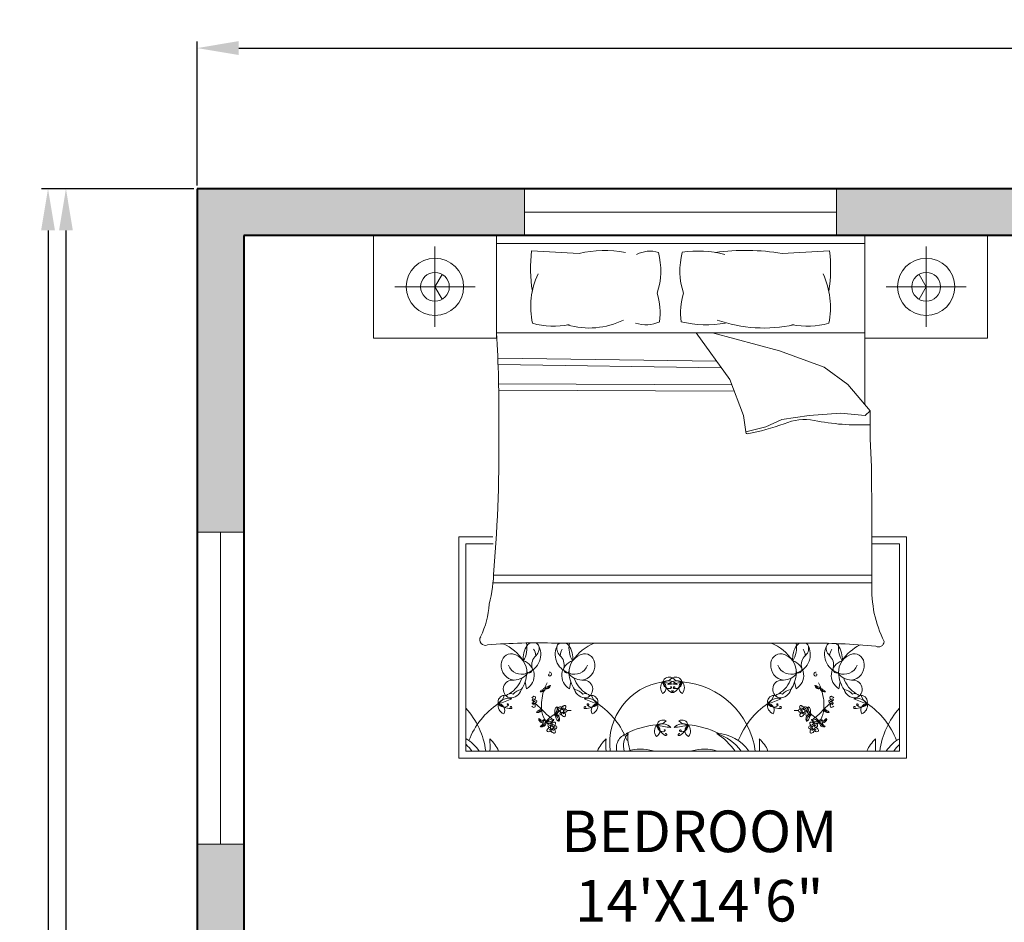
# Model space of a CAD drawing. Units: inches. Extents: x 2138 to 3265, y 2149 to 3392.
# Tile 4 of 13: x 2173 to 2363, y 2589 to 2762. Entities that reach past the tile are written whole.
import ezdxf

# ---------------------------------------------------------------- set-up
doc = ezdxf.new("R2010")
doc.units = ezdxf.units.IN
for name, color, linetype, lineweight in [('A-ANNO-DIMS', 2, 'Continuous', 18), ('A-AREA-IDEN', 7, 'Continuous', 18), ('A-FURN', 8, 'Continuous', 18), ('A-GLAZ', 150, 'Continuous', 18), ('A-WALL', 7, 'Continuous', 40), ('A-WALL-PATT', 142, 'Continuous', 13)]:
    doc.layers.add(name, color=color, linetype=linetype, lineweight=lineweight)
doc.styles.get("Standard").update_dxf_attribs({"font": 'arial.ttf'})
doc.dimstyles.new('ISO-25', dxfattribs={"dimtxt": 8, "dimasz": 8, "dimexe": 1.25, "dimexo": 0.625, "dimtad": 0, "dimdec": 1, "dimlunit": 4, "dimtxsty": 'Standard', "dimcen": 2.5, "dimadec": 0, "dimazin": 0, "dimtfac": 1, "dimtdec": 1, "dimtmove": 0, "dimatfit": 3, "dimfxl": 1, "dimarcsym": 0})

# ---------------------------------------------------------------- blocks, each defined once
blk = doc.blocks.new('bed')
for p, q in [((2648.79, 2367.17), (2766.9, 2367.17)), ((2672.41, 2367.17), (2672.41, 2334.75)), ((2743.28, 2365.66), (2672.41, 2365.66)), ((2660.6, 2349.61), (2660.6, 2365.05)), ((2755.09, 2349.61), (2755.09, 2365.05)), ((2668.32, 2357.33), (2652.88, 2357.33)), ((2747.37, 2357.33), (2762.8, 2357.33)), ((2672.41, 2348.51), (2743.28, 2348.51)), ((2688.82, 2345), (2701.7, 2348.51)), ((2704.86, 2348.51), (2698.39, 2339.5)), ((2680.2, 2341.89), (2688.82, 2345)), ((2742.96, 2343.6), (2700.91, 2343.01)), ((2675.66, 2338.54), (2680.2, 2341.89)), ((2742.91, 2342.39), (2700.03, 2341.78)), ((2698.39, 2339.5), (2695.75, 2332.57)), ((2671.35, 2333.52), (2675.66, 2338.54)), ((2742.86, 2337.46), (2697.54, 2337.27)), ((2742.85, 2338.67), (2698, 2338.49)), ((2672.31, 2332.57), (2671.35, 2333.52)), ((2677.09, 2333.04), (2672.31, 2332.57)), ((2683.08, 2332.57), (2677.09, 2333.04)), ((2688.34, 2331.85), (2683.08, 2332.57)), ((2691.45, 2330.41), (2688.34, 2331.85)), ((2695.75, 2332.57), (2695.28, 2329.46)), ((2695.28, 2329.46), (2691.45, 2330.41)), ((2664.38, 2309.27), (2671.06, 2309.27)), ((2664.38, 2266.73), (2664.38, 2309.27)), ((2743.94, 2309.27), (2750.49, 2309.27)), ((2750.49, 2309.27), (2750.49, 2266.73)), ((2671.06, 2307.91), (2665.75, 2307.91)), ((2665.75, 2307.91), (2665.75, 2268.1)), ((2749.12, 2307.91), (2743.91, 2307.91)), ((2749.12, 2268.1), (2749.12, 2307.91)), ((2743.81, 2301.91), (2671.05, 2301.91)), ((2743.93, 2300.44), (2671.05, 2300.44)), ((2731.82, 2288.83), (2683.87, 2288.83)), ((2677.39, 2280.07), (2677.12, 2281.41)), ((2685.64, 2280.07), (2685.9, 2281.41)), ((2729.22, 2280.07), (2728.96, 2281.41)), ((2737.48, 2280.07), (2737.74, 2281.41)), ((2665.75, 2268.1), (2749.12, 2268.1)), ((2750.49, 2266.73), (2664.38, 2266.73))]:
    blk.add_line(p, q)
for points in [[(2672.41, 2347.49), (2648.79, 2347.49), (2648.79, 2367.17)], [(2743.28, 2367.17), (2743.28, 2347.49), (2766.9, 2347.49), (2766.9, 2367.17)], [(2660.6, 2357.33), (2661.98, 2359.72)], [(2755.09, 2357.33), (2753.71, 2359.72)], [(2660.6, 2357.33), (2661.98, 2354.94)], [(2755.09, 2357.33), (2753.71, 2354.94)]]:
    blk.add_lwpolyline(points)
for points in [[(2679.19, 2364.23, 0.074897), (2679.34, 2356.51, -0.472817)], [(2707.29, 2356.08, 0.14099), (2707.53, 2363.95, 0.235245)], [(2712.33, 2356.08, -0.14099), (2712.1, 2363.95, -0.235245)], [(2736.49, 2364.23, -0.074897), (2736.35, 2356.51, 0.472817)], [(2671.11, 2322.71, 0.001242), (2671.05, 2300.3, -0.127202), (2668.68, 2289.13)], [(2743.78, 2302.84, 0.056112), (2744.64, 2296.34, 0.095341), (2746.3, 2290.08)]]:
    blk.add_lwpolyline(points, format="xyb")
for centre, radius in [((2660.6, 2357.33), 5.51), ((2755.09, 2357.33), 5.51), ((2660.6, 2357.33), 2.76), ((2755.09, 2357.33), 2.76), ((2684.21, 2275.79), 0.301), ((2730.65, 2275.79), 0.301), ((2682.24, 2272.62), 0.301), ((2732.62, 2272.62), 0.301)]:
    blk.add_circle(centre, radius)
for centre, radius, start, end in [((2744.3, 3488.25), 1125.9, 266.68521, 267.14978), ((2695.38, 2321.49), 42.84, 82.2196, 99.497), ((2704.43, 2343.14), 21.05, 81.5249, 103.96), ((2713.72, 2358.34), 5.84, 63.3437, 106.1026), ((2722.48, 2343.56), 20.76, 76.3427, 101.1841), ((2671.39, 3488.25), 1125.9, 272.85022, 273.31479), ((2694.24, 2353.42), 15.22, 155.1316, 191.7583), ((2721.45, 2353.42), 15.22, 348.2417, 24.8684), ((2693.37, 2352.14), 14.47, 354.0129, 15.8293), ((2726.26, 2352.14), 14.47, 164.1707, 185.9871), ((2691.74, 2376.86), 27.45, 258.0397, 289.2615), ((2702.85, 2370.87), 20.83, 259.8617, 283.6238), ((2714.51, 2356.3), 6.26, 245.0183, 288.5407), ((2725.45, 2364.44), 15.03, 243.8761, 286.1746), ((2683.41, 2365.61), 15.83, 255.1039, 281.0369), ((2732.28, 2365.61), 15.83, 258.9631, 284.8961), ((2955.01, 2334.07), 212.22, 176.1, 180.9282), ((2563.06, 2330.59), 108.33, 355.8294, 1.553), ((2673.37, 2375.35), 44.58, 267.4519, 281.3392), ((2684.03, 2322.21), 9.61, 66.2616, 101.3392), ((2703.48, 2374.09), 45.8, 250.1194, 259.3383), ((3019.62, 2326.36), 276.84, 179.1145, 184.8735), ((2695.01, 2329.36), 0.285, 268.8623, 19.7536), ((2745.4, 2289.48), 1.08, 246.5219, 33.8264), ((2669.77, 2289.2), 1.09, 183.98, 297.3412), ((2682.46, 2165.89), 122.95, 89.3433, 95.6887), ((2669.31, 2280.52), 8.94, 33.6671, 63.2997), ((2681.29, 2285.83), 4.56, 145.785, 184.7304), ((2672.59, 2287.96), 4.89, 328.8218, 9.1554), ((2678.65, 2287.53), 1.42, 120.0293, 142.325), ((2676.38, 2286.69), 3.76, 289.2822, 29.1751), ((2678.05, 2287.81), 1.77, 311.5653, 23.8354), ((2678.65, 2287.53), 1.42, 44.4517, 63.558), ((2686.65, 2286.69), 3.76, 150.8249, 250.7178), ((2684.98, 2287.81), 1.77, 156.1646, 228.4347), ((2684.38, 2287.53), 1.42, 113.229, 135.5483), ((2684.38, 2287.53), 1.42, 37.675, 66.7144), ((2681.74, 2285.83), 4.56, 355.2696, 34.215), ((2690.44, 2287.96), 4.89, 169.7133, 211.1782), ((2693.72, 2280.52), 8.94, 111.4941, 146.3329), ((2721.15, 2280.52), 8.94, 33.6671, 68.5059), ((2733.13, 2285.83), 4.56, 145.785, 184.7304), ((2724.42, 2287.96), 4.89, 328.8218, 10.2867), ((2730.49, 2287.53), 1.42, 113.2856, 142.325), ((2728.21, 2286.69), 3.76, 289.2822, 29.1751), ((2730.49, 2287.53), 1.42, 44.4517, 66.7144), ((2729.88, 2287.81), 1.77, 311.5653, 23.8354), ((2735.44, 2173.96), 114.93, 85.2402, 91.8035), ((2738.49, 2286.69), 3.76, 150.8249, 250.7178), ((2736.82, 2287.81), 1.77, 156.1646, 228.4347), ((2736.22, 2287.53), 1.42, 106.6343, 135.5483), ((2736.22, 2287.53), 1.42, 37.675, 72.5814), ((2733.57, 2285.83), 4.56, 355.2696, 34.215), ((2742.28, 2287.96), 4.89, 169.249, 211.1782), ((2745.56, 2280.52), 8.94, 113.6453, 146.3329), ((2674.52, 2284.81), 1.99, 84.4856, 181.0538), ((2673.9, 2283.33), 3.55, 355.2933, 76.921), ((2680.83, 2284.67), 2.42, 131.5653, 195.1471), ((2675.81, 2286.01), 3.4, 7.436, 29.9149), ((2682.2, 2284.67), 2.42, 344.8529, 48.4347), ((2687.22, 2286.01), 3.4, 150.0851, 172.564), ((2689.12, 2283.33), 3.55, 103.079, 184.7067), ((2688.51, 2284.81), 1.99, 358.9462, 95.5144), ((2726.35, 2284.81), 1.99, 84.4856, 181.0538), ((2725.74, 2283.33), 3.55, 355.2933, 76.921), ((2732.66, 2284.67), 2.42, 131.5653, 195.1471), ((2727.65, 2286.01), 3.4, 7.436, 29.9149), ((2734.04, 2284.67), 2.42, 344.8529, 48.4347), ((2739.05, 2286.01), 3.4, 150.0851, 172.564), ((2740.96, 2283.33), 3.55, 103.079, 184.7067), ((2740.35, 2284.81), 1.99, 358.9462, 95.5144), ((2675.33, 2284.52), 2.82, 174.9449, 262.8857), ((2676.44, 2285.59), 2.74, 201.5819, 291.4221), ((2675.92, 2282.62), 2.94, 299.9085, 73.1337), ((2687.1, 2282.62), 2.94, 106.8663, 240.0915), ((2686.58, 2285.59), 2.74, 248.5779, 338.4181), ((2687.69, 2284.52), 2.82, 277.1143, 5.0551), ((2727.17, 2284.52), 2.82, 174.9449, 262.8857), ((2728.28, 2285.59), 2.74, 201.5819, 291.4221), ((2727.76, 2282.62), 2.94, 299.9085, 73.1337), ((2738.94, 2282.62), 2.94, 106.8663, 240.0915), ((2738.42, 2285.59), 2.74, 248.5779, 338.4181), ((2739.53, 2284.52), 2.82, 277.1143, 5.0551), ((2674.84, 2285.15), 3.43, 272.3591, 324.0401), ((2671.12, 2283.43), 6.34, 326.2883, 356.5076), ((2681.29, 2285.83), 4.56, 212.7011, 216.3445), ((2677.78, 2283.85), 0.733, 257.3041, 15.1471), ((2681.85, 2282.74), 0.228, 102.7051, 280.4384), ((2681.83, 2282.88), 0.37, 280.4384, 100.4136), ((2685.25, 2283.85), 0.733, 164.8529, 282.6959), ((2681.74, 2285.83), 4.56, 323.6555, 327.2989), ((2688.18, 2285.15), 3.43, 215.9599, 267.6409), ((2691.91, 2283.43), 6.34, 183.4924, 213.7117), ((2708.79, 2281.04), 1.28, 63.0274, 163.8037), ((2710.01, 2281.04), 1.28, 16.1963, 116.9726), ((2726.68, 2285.15), 3.43, 272.3591, 324.0401), ((2722.96, 2283.43), 6.34, 326.2883, 356.5076), ((2733.13, 2285.83), 4.56, 212.7011, 216.3445), ((2729.62, 2283.85), 0.733, 257.3041, 15.1471), ((2733.04, 2282.88), 0.37, 79.5864, 259.5616), ((2733.01, 2282.74), 0.228, 259.5616, 77.2949), ((2737.08, 2283.85), 0.733, 164.8529, 282.6959), ((2733.57, 2285.83), 4.56, 323.6555, 327.2989), ((2740.02, 2285.15), 3.43, 215.9599, 267.6409), ((2743.75, 2283.43), 6.34, 183.4924, 213.7117), ((2674.68, 2279.97), 1.77, 80.264, 250.8688), ((2671.17, 2283.88), 5.58, 301.2614, 341.7045), ((2690.04, 2276.79), 9.78, 153.0032, 159.8941), ((2681.22, 2280.14), 0.241, 84.3784, 186.0543), ((2680.74, 2282.21), 1.9, 285.5129, 293.6099), ((2681.98, 2280.07), 0.62, 87.3579, 140.4944), ((2680.54, 2281.85), 1.87, 301.164, 321.5612), ((2679.02, 2282.18), 3.33, 324.6898, 333.4936), ((2691.86, 2283.88), 5.58, 198.2955, 238.7386), ((2688.34, 2279.97), 1.77, 289.1312, 99.736), ((2708.76, 2266.02), 15.42, 94.4623, 172.255), ((2708.83, 2280.25), 1.71, 137.7873, 219.1145), ((2706.89, 2280.3), 1.29, 298.5391, 58.3627), ((2707.5, 2284.03), 2.63, 271.4585, 315.3727), ((2708.57, 2279.17), 2.44, 45.5411, 114.3101), ((2710.79, 2291.69), 10.79, 252.593, 267.2582), ((2708.82, 2281.35), 1.26, 177.7585, 283.852), ((2711.25, 2282.66), 3.9, 198.9159, 238.011), ((2710.23, 2279.17), 2.44, 65.6899, 134.4589), ((2708.01, 2291.69), 10.79, 272.7418, 287.407), ((2709.09, 2280.28), 0.167, 283.852, 219.9245), ((2711.31, 2284.03), 2.63, 224.6273, 268.5415), ((2709.7, 2280.35), 0.101, 320.1909, 256.0209), ((2707.55, 2282.66), 3.9, 301.989, 341.0841), ((2709.98, 2281.35), 1.26, 256.148, 2.2415), ((2711.91, 2280.3), 1.29, 121.6373, 241.4609), ((2709.97, 2280.25), 1.71, 320.8855, 42.2127), ((2709.54, 2269.58), 11.94, 352.8636, 81.8197), ((2726.52, 2279.97), 1.77, 80.264, 250.8688), ((2723.01, 2283.88), 5.58, 301.2614, 341.7045), ((2734.32, 2281.85), 1.87, 218.4388, 238.836), ((2732.89, 2280.07), 0.62, 39.5056, 92.6421), ((2735.84, 2282.18), 3.33, 206.5064, 215.3102), ((2734.13, 2282.21), 1.9, 246.3901, 254.4871), ((2724.82, 2276.79), 9.78, 20.1059, 26.9968), ((2733.64, 2280.14), 0.241, 353.9457, 95.6216), ((2743.69, 2283.88), 5.58, 198.2955, 238.7386), ((2740.18, 2279.97), 1.77, 289.1312, 99.736), ((2673.18, 2277.52), 1.28, 92.9516, 193.728), ((2670.57, 2279.47), 2.63, 301.3827, 345.2969), ((2674.32, 2278.05), 1.09, 63.9755, 143.2681), ((2674.26, 2280.51), 2.21, 265.969, 344.3045), ((2676.64, 2277.57), 2.36, 96.1662, 141.5825), ((2678.79, 2278.04), 0.502, 101.5637, 142.6358), ((2678.88, 2278.4), 0.232, 345.2356, 144.9248), ((2680.55, 2279.22), 0.62, 101.3256, 154.4621), ((2679.66, 2281.32), 1.87, 280.2588, 300.656), ((2680.09, 2282.82), 3.33, 268.3264, 277.1302), ((2690.04, 2276.79), 9.78, 163.5842, 183.8277), ((2679.25, 2281.32), 1.9, 308.2101, 316.3071), ((2680.42, 2280.07), 0.567, 278.3432, 4.2869), ((2680.1, 2280.57), 0.99, 300.656, 332.6341), ((2680.85, 2279.92), 0.241, 55.7657, 157.4417), ((2681, 2281.1), 0.99, 269.1859, 301.164), ((2681.29, 2280.59), 0.567, 237.5332, 323.4768), ((2686.38, 2277.57), 2.36, 38.4175, 83.8338), ((2688.77, 2280.51), 2.21, 195.6955, 274.031), ((2688.71, 2278.05), 1.09, 36.7319, 116.0245), ((2689.84, 2277.52), 1.28, 346.272, 87.0484), ((2692.46, 2279.47), 2.63, 194.7031, 238.6173), ((2709.29, 2279.51), 0.192, 238.011, 71.5592), ((2709.32, 2279.61), 0.093, 71.5592, 188.0167), ((2709.51, 2279.51), 0.192, 108.4408, 301.989), ((2709.48, 2279.61), 0.093, 351.9833, 108.4408), ((2725.02, 2277.52), 1.28, 92.9516, 193.728), ((2722.41, 2279.47), 2.63, 301.3827, 345.2969), ((2726.16, 2278.05), 1.09, 63.9755, 143.2681), ((2726.1, 2280.51), 2.21, 265.969, 344.3045), ((2728.48, 2277.57), 2.36, 96.1662, 141.5825), ((2733.58, 2280.59), 0.567, 216.5232, 302.4668), ((2733.87, 2281.1), 0.99, 238.836, 270.8141), ((2734.02, 2279.92), 0.241, 22.5583, 124.2343), ((2734.45, 2280.07), 0.567, 175.7131, 261.6568), ((2734.76, 2280.57), 0.99, 207.3659, 239.344), ((2724.82, 2276.79), 9.78, 356.1723, 16.4158), ((2735.61, 2281.32), 1.9, 223.6929, 231.7899), ((2735.21, 2281.32), 1.87, 239.344, 259.7412), ((2734.78, 2282.82), 3.33, 262.8698, 271.6736), ((2734.32, 2279.22), 0.62, 25.5379, 78.6744), ((2735.98, 2278.4), 0.232, 35.0752, 194.7644), ((2736.07, 2278.04), 0.502, 37.3642, 78.4363), ((2740.6, 2280.51), 2.21, 195.6955, 274.031), ((2738.22, 2277.57), 2.36, 38.4175, 83.8338), ((2740.54, 2278.05), 1.09, 36.7319, 116.0245), ((2744.29, 2279.47), 2.63, 194.7031, 238.6173), ((2741.68, 2277.52), 1.28, 346.272, 87.0484), ((2680.65, 2264.49), 15.42, 124.3865, 158.5908), ((2673.61, 2276.86), 1.71, 167.7115, 249.0387), ((2673.92, 2275.8), 2.44, 75.4653, 144.2343), ((2669.6, 2287.75), 10.79, 282.5173, 297.1824), ((2671.9, 2275.93), 1.29, 328.4633, 88.2869), ((2674.51, 2280.16), 3.9, 228.8402, 267.9352), ((2673.06, 2277.81), 1.26, 207.6827, 313.7762), ((2673.82, 2277.02), 0.167, 313.7762, 249.7183), ((2674.35, 2276.55), 0.093, 101.4834, 217.9409), ((2674.37, 2276.45), 0.192, 267.9352, 101.4834), ((2678.38, 2277.58), 0.301, 273.2768, 86.7232), ((2678.79, 2277.02), 0.497, 217.7621, 259.0403), ((2678.73, 2277.86), 0.287, 91.1081, 181.8675), ((2679.32, 2277.68), 0.913, 203.4276, 227.6104), ((2679.03, 2277.29), 0.622, 80.3487, 133.6538), ((2678.92, 2277.8), 0.492, 229.7889, 317.6792), ((2678.39, 2278.44), 0.723, 288.7263, 352.5032), ((2678.37, 2276.76), 0.699, 355.053, 68.3618), ((2678.92, 2276.64), 0.985, 83.0852, 105.7171), ((2678.83, 2276.72), 0.231, 232.4737, 355.053), ((2672.1, 2268.47), 11.21, 43.1541, 52.0459), ((2679.1, 2277.64), 0.259, 317.6792, 80.3487), ((2681.91, 2276.24), 1.37, 304.5369, 16.3699), ((2683.81, 2275.85), 0.97, 127.3105, 187.9252), ((2682.48, 2275.96), 0.996, 355.0106, 41.658), ((2683.88, 2276.21), 0.41, 126.1046, 271.4281), ((2683.83, 2276.32), 0.295, 353.7526, 131.7054), ((2684.63, 2276.26), 0.502, 101.5637, 176.365), ((2684.22, 2276.65), 0.723, 288.7263, 352.5032), ((2684.72, 2276.61), 0.232, 345.2356, 144.9248), ((2688.65, 2276.45), 0.192, 78.5166, 272.0648), ((2689.11, 2275.8), 2.44, 35.7657, 104.5347), ((2693.42, 2287.75), 10.79, 242.8176, 257.4827), ((2688.52, 2280.16), 3.9, 272.0648, 311.1598), ((2688.67, 2276.55), 0.093, 322.0591, 78.5166), ((2689.97, 2277.81), 1.26, 226.2238, 332.3173), ((2689.23, 2277.08), 0.101, 290.2667, 226.2271), ((2691.12, 2275.93), 1.29, 91.7131, 211.5367), ((2689.41, 2276.86), 1.71, 290.9613, 12.2885), ((2682.38, 2264.49), 15.42, 21.4092, 55.6135), ((2732.49, 2264.49), 15.42, 124.3865, 158.5908), ((2725.45, 2276.86), 1.71, 167.7115, 249.0387), ((2725.76, 2275.8), 2.44, 75.4653, 144.2343), ((2721.44, 2287.75), 10.79, 282.5173, 297.1824), ((2724.9, 2277.81), 1.26, 207.6827, 313.7762), ((2726.35, 2280.16), 3.9, 228.8402, 267.9352), ((2723.74, 2275.93), 1.29, 328.4633, 88.2869), ((2725.65, 2277.02), 0.167, 313.7762, 249.7183), ((2726.19, 2276.55), 0.093, 101.4834, 217.9409), ((2726.21, 2276.45), 0.192, 267.9352, 101.4834), ((2730.15, 2276.61), 0.232, 35.0752, 194.7644), ((2730.64, 2276.65), 0.723, 187.4968, 251.2737), ((2730.24, 2276.26), 0.502, 3.635, 78.4363), ((2731.03, 2276.32), 0.295, 48.2946, 186.2474), ((2730.99, 2276.21), 0.41, 268.5719, 53.8954), ((2732.39, 2275.96), 0.996, 138.342, 184.9894), ((2732.96, 2276.24), 1.37, 163.6301, 235.4631), ((2731.05, 2275.85), 0.97, 352.0748, 52.6895), ((2742.77, 2268.47), 11.21, 127.9541, 136.8459), ((2735.77, 2277.64), 0.259, 99.6513, 222.3208), ((2735.94, 2277.8), 0.492, 222.3208, 310.2111), ((2735.83, 2277.29), 0.622, 46.3462, 99.6513), ((2736.47, 2278.44), 0.723, 187.4968, 251.2737), ((2736.5, 2276.76), 0.699, 111.6382, 184.947), ((2736.03, 2276.72), 0.231, 184.947, 307.5263), ((2735.95, 2276.64), 0.985, 74.2829, 96.9148), ((2736.13, 2277.86), 0.287, 358.1325, 88.8919), ((2735.54, 2277.68), 0.913, 312.3896, 336.5724), ((2736.08, 2277.02), 0.497, 280.9597, 322.2379), ((2736.49, 2277.58), 0.301, 93.2768, 266.7232), ((2740.49, 2276.45), 0.192, 78.5166, 272.0648), ((2740.94, 2275.8), 2.44, 35.7657, 104.5347), ((2745.26, 2287.75), 10.79, 242.8176, 257.4827), ((2740.36, 2280.16), 3.9, 272.0648, 311.1598), ((2740.51, 2276.55), 0.093, 322.0591, 78.5166), ((2741.81, 2277.81), 1.26, 226.2238, 332.3173), ((2741.07, 2277.08), 0.101, 290.2667, 226.2271), ((2742.96, 2275.93), 1.29, 91.7131, 211.5367), ((2741.25, 2276.86), 1.71, 290.9613, 12.2885), ((2734.21, 2264.49), 15.42, 21.4092, 55.6135), ((2654.26, 2266.02), 15.42, 7.745, 41.8856), ((2679.84, 2275.25), 0.62, 101.3256, 154.4621), ((2678.95, 2277.35), 1.87, 280.2588, 300.656), ((2679.38, 2278.84), 3.33, 268.3264, 277.1302), ((2678.55, 2277.34), 1.9, 308.2101, 316.3071), ((2679.71, 2276.1), 0.567, 278.3432, 4.2869), ((2679.4, 2276.6), 0.99, 300.656, 332.6341), ((2680.14, 2275.94), 0.241, 55.7657, 157.4417), ((2685.17, 2276.55), 4.9, 184.756, 209.2041), ((2692.23, 2286.99), 16.14, 222.2412, 232.1744), ((2685.67, 2270.03), 5.88, 120.544, 139.818), ((2682.64, 2275.93), 0.833, 272.8499, 356.1226), ((2682.05, 2275.61), 0.807, 321.7607, 7.9252), ((2682.22, 2274.45), 0.807, 8.7227, 54.8872), ((2682.26, 2273.8), 1.37, 0.278, 72.111), ((2682.88, 2274.31), 0.833, 20.5253, 88.5375), ((2683.58, 2275.23), 0.298, 148.0499, 225.6268), ((2685.67, 2270.03), 5.88, 113.0501, 113.8477), ((2684.13, 2274.88), 0.948, 104.7558, 148.0499), ((2683.6, 2275.56), 0.594, 247.4086, 351.4386), ((2683.76, 2275.54), 0.199, 262.906, 7.132), ((2683.55, 2275.97), 0.414, 0.0645, 61.1507), ((2683.65, 2276.32), 0.473, 311.8413, 355.7877), ((2684.62, 2275.23), 0.497, 151.2196, 259.0403), ((2684.56, 2276.08), 0.287, 91.1081, 181.8675), ((2685.16, 2275.9), 0.913, 203.4276, 227.6104), ((2684.87, 2275.5), 0.622, 80.3487, 133.6538), ((2684.75, 2276.01), 0.492, 229.7889, 317.6792), ((2684.2, 2274.97), 0.699, 355.053, 68.3618), ((2684.75, 2274.85), 0.985, 83.0852, 105.7171), ((2684.67, 2274.93), 0.231, 232.4737, 355.053), ((2684.93, 2275.86), 0.259, 317.6792, 80.3487), ((2685.67, 2270.03), 5.88, 87.1071, 94.7585), ((2729.19, 2270.03), 5.88, 85.2415, 92.8929), ((2729.94, 2275.86), 0.259, 99.6513, 222.3208), ((2730.11, 2276.01), 0.492, 222.3208, 310.2111), ((2730, 2275.5), 0.622, 46.3462, 99.6513), ((2730.66, 2274.97), 0.699, 111.6382, 184.947), ((2730.2, 2274.93), 0.231, 184.947, 307.5263), ((2730.12, 2274.85), 0.985, 74.2829, 96.9148), ((2730.3, 2276.08), 0.287, 358.1325, 88.8919), ((2729.71, 2275.9), 0.913, 312.3896, 336.5724), ((2730.24, 2275.23), 0.497, 280.9597, 28.7804), ((2731.27, 2275.56), 0.594, 188.5614, 292.5914), ((2731.21, 2276.32), 0.473, 184.2123, 228.1587), ((2731.31, 2275.97), 0.414, 118.8493, 179.9355), ((2731.1, 2275.54), 0.199, 172.868, 277.094), ((2730.73, 2274.88), 0.948, 31.9501, 75.2442), ((2731.99, 2274.31), 0.833, 91.4625, 159.4747), ((2732.6, 2273.8), 1.37, 107.889, 179.722), ((2732.22, 2275.93), 0.833, 183.8774, 267.1501), ((2731.29, 2275.23), 0.298, 314.3732, 31.9501), ((2729.19, 2270.03), 5.88, 66.1523, 66.9499), ((2732.64, 2274.45), 0.807, 125.1128, 171.2773), ((2732.81, 2275.61), 0.807, 172.0748, 218.2393), ((2729.19, 2270.03), 5.88, 40.182, 59.456), ((2722.64, 2286.99), 16.14, 307.8256, 317.7588), ((2729.7, 2276.55), 4.9, 330.7959, 355.244), ((2735.15, 2276.1), 0.567, 175.7131, 261.6568), ((2734.72, 2275.94), 0.241, 22.5583, 124.2343), ((2735.46, 2276.6), 0.99, 207.3659, 239.344), ((2736.32, 2277.34), 1.9, 223.6929, 231.7899), ((2735.91, 2277.35), 1.87, 239.344, 259.7412), ((2735.48, 2278.84), 3.33, 262.8698, 271.6736), ((2735.02, 2275.25), 0.62, 25.5379, 78.6744), ((2760.6, 2266.02), 15.42, 138.1144, 172.255), ((2680.05, 2274.16), 0.336, 146.8636, 236.9021), ((2684.79, 2281.56), 8.79, 235.1882, 238.8844), ((2680.63, 2274.64), 0.909, 199.4799, 267.6828), ((2680.53, 2274.3), 0.783, 212.8155, 277.3992), ((2680.07, 2273.78), 0.909, 266.9701, 338.2913), ((2675.28, 2280.27), 8.79, 302.6784, 306.3746), ((2680.3, 2273.06), 0.336, 214.3538, 304.3923), ((2680.43, 2274.33), 0.348, 238.8844, 314.2646), ((2680.35, 2273.55), 0.783, 280.3057, 17.1958), ((2680.29, 2273.47), 0.348, 306.3746, 21.7548), ((2680.85, 2273.7), 0.262, 19.3605, 201.7548), ((2680.85, 2273.89), 0.262, 311.8703, 134.2646), ((2685.79, 2271.5), 5.24, 153.7819, 158.2913), ((2681.62, 2275.08), 1.37, 247.2305, 319.0635), ((2681.16, 2274.62), 0.807, 264.4544, 310.6188), ((2685.17, 2276.55), 4.9, 214.0033, 222.4917), ((2681.75, 2274.3), 0.833, 218.3208, 298.8162), ((2681.91, 2273.04), 0.41, 126.1046, 271.4281), ((2681.86, 2273.15), 0.295, 353.7526, 131.7054), ((2682.32, 2273.27), 0.97, 70.0041, 130.6188), ((2681.59, 2272.8), 0.414, 0.0645, 61.1507), ((2681.69, 2273.15), 0.473, 311.8413, 355.7877), ((2681.69, 2274.45), 0.996, 297.7043, 344.3516), ((2682.66, 2273.09), 0.502, 101.5637, 176.365), ((2682.59, 2272.91), 0.287, 91.1081, 181.8675), ((2682.9, 2272.33), 0.622, 80.3487, 133.6538), ((2682.26, 2273.48), 0.723, 288.7263, 352.5032), ((2682.75, 2273.44), 0.232, 345.2356, 144.9248), ((2682.96, 2272.68), 0.259, 317.6792, 80.3487), ((2683.98, 2274.72), 0.97, 188.7227, 249.3375), ((2682.73, 2274.23), 0.996, 334.9899, 21.6373), ((2707.58, 2257.76), 15.42, 94.4623, 117.4146), ((2707.65, 2271.98), 1.71, 137.7873, 219.1145), ((2705.71, 2272.04), 1.29, 298.5391, 58.3627), ((2707.61, 2272.78), 1.28, 63.0274, 163.8037), ((2706.31, 2275.77), 2.63, 271.4585, 315.3727), ((2707.39, 2270.91), 2.44, 45.5411, 114.3101), ((2710.07, 2274.4), 3.9, 198.9159, 238.011), ((2709.61, 2283.43), 10.79, 252.593, 267.2582), ((2707.64, 2273.08), 1.26, 177.7585, 283.852), ((2711.42, 2270.91), 2.44, 65.6899, 134.4589), ((2709.19, 2283.43), 10.79, 272.7418, 287.407), ((2711.19, 2272.78), 1.28, 16.1963, 116.9726), ((2712.49, 2275.77), 2.63, 224.6273, 268.5415), ((2708.73, 2274.4), 3.9, 301.989, 341.0841), ((2711.16, 2273.08), 1.26, 256.148, 2.2415), ((2713.1, 2272.04), 1.29, 121.6373, 241.4609), ((2711.15, 2271.98), 1.71, 320.8855, 42.2127), ((2711.22, 2257.76), 15.42, 62.5854, 85.5377), ((2732.13, 2274.23), 0.996, 158.3627, 205.0101), ((2730.89, 2274.72), 0.97, 290.6625, 351.2773), ((2731.91, 2272.68), 0.259, 99.6513, 222.3208), ((2731.97, 2272.33), 0.622, 46.3462, 99.6513), ((2732.12, 2273.44), 0.232, 35.0752, 194.7644), ((2732.61, 2273.48), 0.723, 187.4968, 251.2737), ((2732.54, 2273.27), 0.97, 49.3812, 109.9959), ((2733.25, 2275.08), 1.37, 220.9365, 292.7695), ((2733.17, 2274.45), 0.996, 195.6484, 242.2957), ((2732.27, 2272.91), 0.287, 358.1325, 88.8919), ((2732.21, 2273.09), 0.502, 3.635, 78.4363), ((2733, 2273.15), 0.295, 48.2946, 186.2474), ((2733.11, 2274.3), 0.833, 241.1838, 321.6792), ((2733.18, 2273.15), 0.473, 184.2123, 228.1587), ((2733.28, 2272.8), 0.414, 118.8493, 179.9355), ((2732.95, 2273.04), 0.41, 268.5719, 53.8954), ((2733.7, 2274.62), 0.807, 229.3812, 275.5456), ((2729.7, 2276.55), 4.9, 317.5083, 325.9967), ((2734.51, 2273.55), 0.783, 162.8042, 259.6943), ((2734.01, 2273.89), 0.262, 45.7354, 228.1297), ((2734.01, 2273.7), 0.262, 338.2452, 160.6395), ((2729.08, 2271.5), 5.24, 21.7087, 26.2181), ((2734.79, 2273.78), 0.909, 201.7087, 273.0299), ((2734.44, 2274.33), 0.348, 225.7354, 301.1156), ((2734.34, 2274.3), 0.783, 262.6008, 327.1845), ((2734.58, 2273.47), 0.348, 158.2452, 233.6254), ((2734.23, 2274.64), 0.909, 272.3172, 340.5201), ((2739.58, 2280.27), 8.79, 233.6254, 237.3216), ((2734.56, 2273.06), 0.336, 235.6077, 325.6462), ((2730.07, 2281.56), 8.79, 301.1156, 304.8118), ((2734.81, 2274.16), 0.336, 303.0979, 33.1364), ((2681.61, 2272.06), 0.298, 148.0499, 225.6268), ((2682.16, 2271.71), 0.948, 104.7558, 148.0499), ((2681.63, 2272.39), 0.594, 247.4086, 351.4386), ((2681.8, 2272.37), 0.199, 262.906, 7.132), ((2682.65, 2272.06), 0.497, 151.2196, 259.0403), ((2683.19, 2272.72), 0.913, 203.4276, 227.6104), ((2682.79, 2272.84), 0.492, 229.7889, 317.6792), ((2682.23, 2271.8), 0.699, 355.053, 68.3618), ((2682.78, 2271.68), 0.985, 83.0852, 105.7171), ((2682.7, 2271.76), 0.231, 232.4737, 355.053), ((2701.02, 2263.95), 7.52, 91.272, 146.5383), ((2703.73, 2262.55), 9.37, 107.8504, 143.6964), ((2708.65, 2259.92), 13.93, 124.0123, 144.053), ((2707.9, 2272.02), 0.167, 283.852, 219.9245), ((2708.11, 2271.25), 0.192, 238.011, 71.5592), ((2708.14, 2271.35), 0.093, 71.5592, 188.0167), ((2710.69, 2271.25), 0.192, 108.4408, 301.989), ((2710.66, 2271.35), 0.093, 351.9833, 108.4408), ((2710.88, 2272.09), 0.101, 320.1909, 256.0209), ((2711.08, 2270.67), 6.91, 338.117, 6.6195), ((2717.42, 2268.75), 2.77, 346.3898, 79.0739), ((2715.34, 2269.13), 3.5, 342.8609, 41.9049), ((2732.08, 2272.84), 0.492, 222.3208, 310.2111), ((2732.63, 2271.8), 0.699, 111.6382, 184.947), ((2732.17, 2271.76), 0.231, 184.947, 307.5263), ((2732.08, 2271.68), 0.985, 74.2829, 96.9148), ((2731.68, 2272.72), 0.913, 312.3896, 336.5724), ((2732.21, 2272.06), 0.497, 280.9597, 28.7804), ((2733.23, 2272.39), 0.594, 188.5614, 292.5914), ((2733.07, 2272.37), 0.199, 172.868, 277.094), ((2732.7, 2271.71), 0.948, 31.9501, 75.2442), ((2733.25, 2272.06), 0.298, 314.3732, 31.9501), ((2662, 2263.95), 7.52, 33.4617, 60.1116), ((2659.3, 2262.55), 9.37, 36.3036, 46.4814), ((2666.21, 2265.69), 6.27, 22.5547, 48.9546), ((2649.03, 2269.06), 21.34, 357.4081, 3.6519), ((2696.82, 2265.69), 6.27, 131.0454, 157.4453), ((2713.99, 2269.06), 21.34, 176.3481, 182.5919), ((2700.87, 2269.06), 21.34, 357.4081, 3.6519), ((2718.05, 2265.69), 6.27, 22.5547, 48.9546), ((2748.65, 2265.69), 6.27, 131.0454, 157.4453), ((2765.83, 2269.06), 21.34, 176.3481, 182.5919), ((2752.86, 2263.95), 7.52, 119.8884, 146.5383), ((2755.57, 2262.55), 9.37, 133.5186, 143.6964), ((2703.27, 2259.99), 8.48, 73.5431, 107.0202), ((2706.63, 2255.62), 12.54, 94.3787, 95.6357), ((2713.23, 2247.02), 22.41, 109.7217, 109.9028), ((2715.53, 2259.99), 8.48, 72.9798, 106.4569), ((2712.17, 2255.62), 12.54, 84.3643, 85.6213), ((2705.57, 2247.02), 22.41, 70.0972, 70.2783)]:
    blk.add_arc(centre, radius, start, end)
blk = doc.blocks.new('*D18')
at = {"layer": 'A-ANNO-DIMS', "color": 0, "lineweight": -2, "transparency": 16777216}
for p, q in [((2207.53, 2730.29), (2207.53, 2757.96)), ((2591.53, 2730.29), (2591.53, 2757.96)), ((2215.53, 2756.71), (2392.12, 2756.71)), ((2583.53, 2756.71), (2406.94, 2756.71))]:
    blk.add_line(p, q, dxfattribs=at)
at = {"layer": 'A-ANNO-DIMS', "color": 0, "transparency": 16777216}
for points in [[(2215.53, 2758.05), (2215.53, 2755.38), (2207.53, 2756.71)], [(2583.53, 2758.05), (2583.53, 2755.38), (2591.53, 2756.71)]]:
    blk.add_solid(points, dxfattribs=at)
at = {"layer": 'Defpoints', "color": 0, "transparency": 16777216}
for p in [(2591.53, 2756.71), (2207.53, 2729.66), (2591.53, 2729.66)]:
    blk.add_point(p, dxfattribs=at)
at = {"layer": 'A-ANNO-DIMS', "color": 0, "transparency": 16777216, "insert": (2399.53, 2756.71), "char_height": 8, "attachment_point": 5}
blk.add_mtext("32'", dxfattribs=at)
blk = doc.blocks.new('*D19')
at = {"layer": 'A-ANNO-DIMS', "color": 0, "lineweight": -2, "transparency": 16777216}
for p, q in [((2206.9, 2729.66), (2181.05, 2729.66)), ((2182.3, 2721.66), (2182.3, 2497.24)), ((2182.3, 2257.66), (2182.3, 2482.09)), ((2206.9, 2249.66), (2181.05, 2249.66))]:
    blk.add_line(p, q, dxfattribs=at)
at = {"layer": 'A-ANNO-DIMS', "color": 0, "transparency": 16777216}
for points in [[(2180.97, 2721.66), (2183.63, 2721.66), (2182.3, 2729.66)], [(2180.97, 2257.66), (2183.63, 2257.66), (2182.3, 2249.66)]]:
    blk.add_solid(points, dxfattribs=at)
at = {"layer": 'Defpoints', "color": 0, "transparency": 16777216}
for p in [(2207.53, 2729.66), (2182.3, 2249.66), (2207.53, 2249.66)]:
    blk.add_point(p, dxfattribs=at)
at = {"layer": 'A-ANNO-DIMS', "color": 0, "transparency": 16777216, "insert": (2182.3, 2489.66), "char_height": 8, "attachment_point": 5, "rotation": 90}
blk.add_mtext("40'", dxfattribs=at)
blk = doc.blocks.new('GLAZ-SASH-60IN')
for p, q in [((0, 9), (0, 0)), ((60, 9), (60, 0)), ((0, 4.5), (60, 4.5))]:
    blk.add_line(p, q)
blk = doc.blocks.new('*D51')
at = {"layer": 'A-ANNO-DIMS', "color": 0, "lineweight": -2, "transparency": 16777216}
for p, q in [((2206.9, 2729.66), (2177.6, 2729.66)), ((2178.85, 2721.66), (2178.85, 2474.19)), ((2178.85, 2197.66), (2178.85, 2445.13)), ((2206.9, 2189.66), (2177.6, 2189.66))]:
    blk.add_line(p, q, dxfattribs=at)
at = {"layer": 'A-ANNO-DIMS', "color": 0, "transparency": 16777216}
for points in [[(2177.52, 2721.66), (2180.19, 2721.66), (2178.85, 2729.66)], [(2177.52, 2197.66), (2180.19, 2197.66), (2178.85, 2189.66)]]:
    blk.add_solid(points, dxfattribs=at)
at = {"layer": 'Defpoints', "color": 0, "transparency": 16777216}
for p in [(2178.85, 2729.66), (2207.53, 2729.66), (2207.53, 2189.66)]:
    blk.add_point(p, dxfattribs=at)
at = {"layer": 'A-ANNO-DIMS', "color": 0, "transparency": 16777216, "insert": (2178.85, 2459.66), "char_height": 8, "attachment_point": 5, "rotation": 90}
blk.add_mtext('45\'-0"', dxfattribs=at)

msp = doc.modelspace()

# ---------------------------------------------------------------- hatches: boundary and pattern name
at = {"layer": 'A-WALL-PATT'}
h = msp.add_hatch(color=256, dxfattribs=at)
h.dxf.hatch_style = 1
h.paths.add_polyline_path([(2270.53, 2729.66), (2207.53, 2729.66), (2207.53, 2663.66), (2216.53, 2663.66), (2216.53, 2720.66), (2270.53, 2720.66)])
h.paths.add_polyline_path([(2484.36, 2729.66), (2330.53, 2729.66), (2330.53, 2720.66), (2384.53, 2720.66), (2384.53, 2546.66), (2372.53, 2546.66), (2372.53, 2542.16), (2389.03, 2542.16), (2389.03, 2720.66), (2484.36, 2720.66)])
h.paths.add_polyline_path([(2591.53, 2729.66), (2544.36, 2729.66), (2544.36, 2720.66), (2582.53, 2720.66), (2582.53, 2684.66), (2591.53, 2684.66)])
h.paths.add_polyline_path([(2591.53, 2624.66), (2582.53, 2624.66), (2582.53, 2588.66), (2456.53, 2588.66), (2456.53, 2584.16), (2582.53, 2584.16), (2582.53, 2512.16), (2456.53, 2512.16), (2456.53, 2507.66), (2494.03, 2507.66), (2494.03, 2501.66), (2498.53, 2501.66), (2498.53, 2507.66), (2582.53, 2507.66), (2582.53, 2495.66), (2591.53, 2495.66)])
h.paths.add_polyline_path([(2591.53, 2471.66), (2582.53, 2471.66), (2582.53, 2459.66), (2498.53, 2459.66), (2498.53, 2471.66), (2497.72, 2471.66, -0.030629), (2494.03, 2471.44), (2494.03, 2459.66), (2431.08, 2459.66, -0.013128), (2431.03, 2457.77), (2431.03, 2455.16), (2494.03, 2455.16), (2494.03, 2449.16), (2498.53, 2449.16), (2498.53, 2455.16), (2582.53, 2455.16), (2582.53, 2443.16), (2591.53, 2443.16)])
h.paths.add_polyline_path([(2591.53, 2419.16), (2582.53, 2419.16), (2582.53, 2407.16), (2498.53, 2407.16), (2498.53, 2419.16), (2497.72, 2419.16, -0.030629), (2494.03, 2418.94), (2494.03, 2402.66), (2582.53, 2402.66), (2582.53, 2360.66), (2591.53, 2360.66)])
h.paths.add_polyline_path([(2591.53, 2300.66), (2582.53, 2300.66), (2582.53, 2258.66), (2515.78, 2258.66), (2515.78, 2249.66), (2591.53, 2249.66)])
h.paths.add_polyline_path([(2455.78, 2258.66), (2389.03, 2258.66), (2389.03, 2455.16), (2395.03, 2455.16), (2395.03, 2459.66), (2384.53, 2459.66), (2384.53, 2258.66), (2375.53, 2258.66), (2375.53, 2249.66), (2455.78, 2249.66)])
h.paths.add_polyline_path([(2315.53, 2253.24), (2315.53, 2258.66), (2296.03, 2258.66), (2296.03, 2249.66), (2315.53, 2249.66)])
h.paths.add_polyline_path([(2236.03, 2258.66), (2216.53, 2258.66), (2216.53, 2290.16), (2207.53, 2290.16), (2207.53, 2249.66), (2236.03, 2249.66)])
h.paths.add_polyline_path([(2216.53, 2396.66), (2207.53, 2396.66), (2207.53, 2350.16), (2216.53, 2350.16)])
h.paths.add_polyline_path([(2216.53, 2603.66), (2207.53, 2603.66), (2207.53, 2456.66), (2216.53, 2456.66), (2216.53, 2542.16), (2264.53, 2542.16), (2264.53, 2470.16), (2252.53, 2470.16), (2252.53, 2465.66), (2269.03, 2465.66), (2269.03, 2542.16), (2336.48, 2542.16, -0.013128), (2336.53, 2544.05), (2336.53, 2546.66), (2216.53, 2546.66)])

# ---------------------------------------------------------------- linework, layer by layer
at = {"layer": 'A-GLAZ'}
for points in [[(2270.53, 2729.66), (2330.53, 2729.66), (2330.53, 2720.66), (2270.53, 2720.66)], [(2207.53, 2663.66), (2216.53, 2663.66), (2216.53, 2603.66), (2207.53, 2603.66)]]:
    msp.add_lwpolyline(points, close=True, dxfattribs=at)
at = {"layer": 'A-WALL'}
for p, q in [((2591.53, 2729.66), (2207.53, 2729.66)), ((2207.53, 2729.66), (2207.53, 2189.66)), ((2216.53, 2720.66), (2216.53, 2546.66)), ((2384.53, 2720.66), (2216.53, 2720.66))]:
    msp.add_line(p, q, dxfattribs=at)

# ---------------------------------------------------------------- block references
at = {"layer": 'A-FURN', "xscale": -1}
msp.add_blockref('bed', (5008.37, 353.49), dxfattribs=at)
at = {"layer": 'A-GLAZ'}
msp.add_blockref('GLAZ-SASH-60IN', (2270.53, 2720.66), dxfattribs=at)
at = {"layer": 'A-GLAZ', "rotation": 89.99999999999916}
msp.add_blockref('GLAZ-SASH-60IN', (2216.53, 2603.66), dxfattribs=at)

# ---------------------------------------------------------------- texts
at = {"layer": 'A-AREA-IDEN', "insert": (2265.6, 2610.15), "char_height": 8, "attachment_point": 1}
msp.add_mtext_dynamic_manual_height_columns('\\pxqc;BEDROOM\\P14\'X14\'6"', width=77.0226, gutter_width=12.5, heights=[0], dxfattribs=at)

# ---------------------------------------------------------------- dimensions: what is measured, and where the dimension line sits
at = {"layer": 'A-ANNO-DIMS'}
dim = msp.add_linear_dim(base=(2591.53, 2756.71), p1=(2207.53, 2729.66), p2=(2591.53, 2729.66), dimstyle='ISO-25', override={"dimclrd": 0, "dimclre": 0, "dimclrt": 0}, dxfattribs=at)
dim.commit()
dim.dimension.update_dxf_attribs({"geometry": '*D18', "text_midpoint": (2399.53, 2756.71)})
for base, p1, p2, override, picture, middle in [((2178.85, 2729.66), (2207.53, 2189.66), (2207.53, 2729.66), {"dimdec": 1, "dimlfac": 1, "dimrnd": 0, "dimzin": 1, "dimdsep": 46, "dimlunit": 4, "dimfrac": 2}, '*D51', (2178.85, 2459.66)), ((2182.3, 2249.66), (2207.53, 2729.66), (2207.53, 2249.66), {"dimclrd": 0, "dimclre": 0, "dimclrt": 0}, '*D19', (2182.3, 2489.66))]:
    dim = msp.add_linear_dim(base=base, p1=p1, p2=p2, angle=90, dimstyle='ISO-25', override=override, dxfattribs=at)
    dim.commit()
    dim.dimension.update_dxf_attribs({"geometry": picture, "text_midpoint": middle})

doc.saveas('drawing.dxf')
